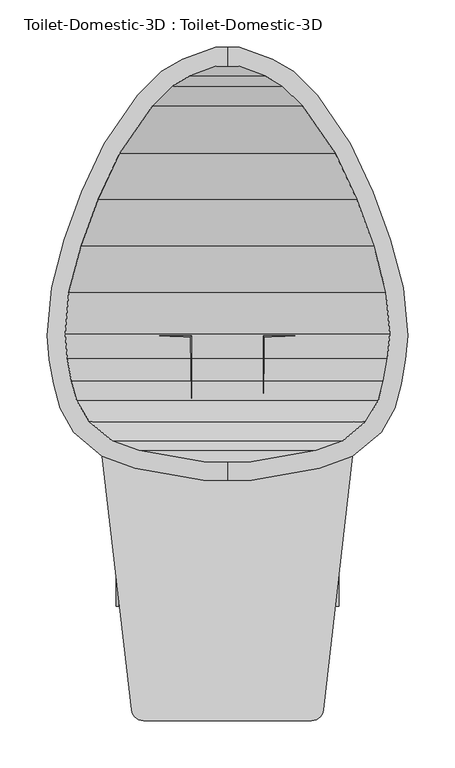
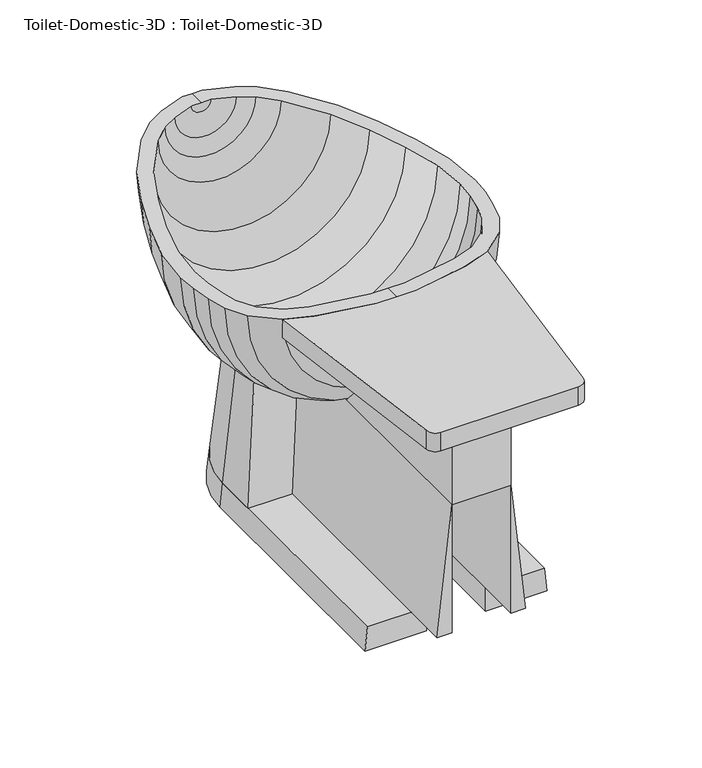
"""IFC4 building model written with IfcOpenShell, lengths in millimetres: flow terminal geometry, Toilet-Domestic-3D : Toilet-Domestic-3D."""

from ifc_helpers import new_model, si_unit, point, frame, frame_2d, origin, place, context, project, spatial, polyline, circle_curve, trimmed, segment, composite_curve, outline, extrude, source, transform, mapped, element, save
from ifc_brep_helpers import plane_surface, revolved_surface, advanced_brep


def toilet_domestic_3d_toilet_domestic_3d_9ecb9d01(model_context):
    return source(origin(), model_context, "Body", "SolidModel", [
        advanced_brep(
        [(-25.4, -152.4, 361.95), (0.0, -152.4, 361.95), (0.0, -133.6394123, 361.95), (-22.0920022, -133.6394123, 361.95), (-94.1172813, -120.9394123, 361.95), (-121.9980886, -110.7916284, 361.95), (-146.1085923, -90.5605136, 361.95), (-159.5484355, -68.2281551, 361.95), (-165.101298, -47.5045901, 361.95), (-169.3087351, -23.6430284, 361.95), (-171.5645445, 2.1409906, 361.95), (-167.7238545, 46.0402777, 361.95), (-154.575847, 95.1093097, 361.95), (-136.654021, 144.3491221, 361.95), (-114.0255101, 192.8761202, 361.95), (-79.2146703, 243.0564036, 361.95), (-58.4178985, 263.8531754, 361.95), (-39.5113323, 274.7688865, 361.95), (-12.5224565, 284.592034, 361.95), (0.0, 284.592034, 361.95), (0.0, 304.8, 361.95), (-12.7, 304.8, 361.95), (-47.5929632, 292.1, 361.95), (-69.5900085, 279.4, 361.95), (-94.9900085, 254.0, 361.95), (-130.2307553, 203.2, 361.95), (-153.9191843, 152.4, 361.95), (-172.4088722, 101.6, 361.95), (-186.0724883, 50.6066907, 361.95), (-190.5, 0.0, 361.95), (-188.2862441, -25.3033453, 361.95), (-183.790496, -50.8, 361.95), (-176.9845865, -76.2, 361.95), (-162.5887836, -101.6, 361.95), (-132.3182423, -127.0, 361.95), (-97.4252791, -139.7, 361.95), (25.4, -152.4, 361.95), (97.4252791, -139.7, 361.95), (132.3182423, -127.0, 361.95), (162.5887836, -101.6, 361.95), (176.9845865, -76.2, 361.95), (183.790496, -50.8, 361.95), (188.2862441, -25.3033453, 361.95), (190.5, 0.0, 361.95), (186.0724883, 50.6066907, 361.95), (172.4088722, 101.6, 361.95), (153.9191843, 152.4, 361.95), (130.2307553, 203.2, 361.95), (94.9900085, 254.0, 361.95), (69.5900085, 279.4, 361.95), (47.5929632, 292.1, 361.95), (12.7, 304.8, 361.95), (12.5224565, 284.592034, 361.95), (39.5113323, 274.7688865, 361.95), (58.4178985, 263.8531754, 361.95), (79.2146703, 243.0564036, 361.95), (114.0255101, 192.8761202, 361.95), (136.654021, 144.3491221, 361.95), (154.575847, 95.1093097, 361.95), (167.7238545, 46.0402777, 361.95), (171.5645445, 2.1409906, 361.95), (169.3087351, -23.6430284, 361.95), (165.101298, -47.5045901, 361.95), (159.5484355, -68.2281551, 361.95), (146.1085923, -90.5605136, 361.95), (121.9980886, -110.7916284, 361.95), (94.1172813, -120.9394123, 361.95), (22.0920022, -133.6394123, 361.95)],
        [
            (0, 1),
            (1, 2),
            (2, 3),
            (3, 4),
            (4, 5),
            (5, 6),
            (6, 7),
            (7, 8),
            (8, 9),
            (9, 10),
            (10, 11),
            (11, 12),
            (12, 13),
            (13, 14),
            (14, 15),
            (15, 16),
            (16, 17),
            (17, 18),
            (18, 19),
            (19, 20),
            (20, 21),
            (21, 22),
            (22, 23),
            (23, 24),
            (24, 25),
            (25, 26),
            (26, 27),
            (27, 28),
            (28, 29),
            (29, 30),
            (30, 31),
            (31, 32),
            (32, 33),
            (33, 34),
            (34, 35),
            (35, 0),
            (36, 37),
            (37, 38),
            (38, 39),
            (39, 40),
            (40, 41),
            (41, 42),
            (42, 43),
            (43, 44),
            (44, 45),
            (45, 46),
            (46, 47),
            (47, 48),
            (48, 49),
            (49, 50),
            (50, 51),
            (51, 20),
            (19, 52),
            (52, 53),
            (53, 54),
            (54, 55),
            (55, 56),
            (56, 57),
            (57, 58),
            (58, 59),
            (59, 60),
            (60, 61),
            (61, 62),
            (62, 63),
            (63, 64),
            (64, 65),
            (65, 66),
            (66, 67),
            (67, 2),
            (1, 36),
            (36, 0, circle_curve(frame((0.0, -152.4, 361.95), z_axis=(0.0, 1.0, 0.0), x_axis=(-1.0, 0.0, 0.0)), 25.4)),
            (35, 37, circle_curve(frame((0.0, -139.7, 361.95), z_axis=(0.0, -1.0, 0.0), x_axis=(-1.0, 0.0, 0.0)), 97.4252791)),
            (34, 38, circle_curve(frame((0.0, -127.0, 361.95), z_axis=(0.0, -1.0, 0.0), x_axis=(-1.0, 0.0, 0.0)), 132.3182423)),
            (33, 39, circle_curve(frame((0.0, -101.6, 361.95), z_axis=(0.0, -1.0, 0.0), x_axis=(-1.0, 0.0, 0.0)), 162.5887836)),
            (32, 40, circle_curve(frame((0.0, -76.2, 361.95), z_axis=(0.0, -1.0, 0.0), x_axis=(-1.0, 0.0, 0.0)), 176.9845865)),
            (31, 41, circle_curve(frame((0.0, -50.8, 361.95), z_axis=(0.0, -1.0, 0.0), x_axis=(-1.0, 0.0, 0.0)), 183.790496)),
            (30, 42, circle_curve(frame((0.0, -25.3033453, 361.95), z_axis=(0.0, -1.0, 0.0), x_axis=(-1.0, 0.0, 0.0)), 188.2862441)),
            (29, 43, circle_curve(frame((0.0, 0.0, 361.95), z_axis=(0.0, -1.0, 0.0), x_axis=(-1.0, 0.0, 0.0)), 190.5)),
            (28, 44, circle_curve(frame((0.0, 50.6066907, 361.95), z_axis=(0.0, -1.0, 0.0), x_axis=(-1.0, 0.0, 0.0)), 186.0724883)),
            (27, 45, circle_curve(frame((0.0, 101.6, 361.95), z_axis=(0.0, -1.0, 0.0), x_axis=(-1.0, 0.0, 0.0)), 172.4088722)),
            (26, 46, circle_curve(frame((0.0, 152.4, 361.95), z_axis=(0.0, -1.0, 0.0), x_axis=(-1.0, 0.0, 0.0)), 153.9191843)),
            (25, 47, circle_curve(frame((0.0, 203.2, 361.95), z_axis=(0.0, -1.0, 0.0), x_axis=(-1.0, 0.0, 0.0)), 130.2307553)),
            (24, 48, circle_curve(frame((0.0, 254.0, 361.95), z_axis=(0.0, -1.0, 0.0), x_axis=(-1.0, 0.0, 0.0)), 94.9900085)),
            (23, 49, circle_curve(frame((0.0, 279.4, 361.95), z_axis=(0.0, -1.0, 0.0), x_axis=(-1.0, 0.0, 0.0)), 69.5900085)),
            (22, 50, circle_curve(frame((0.0, 292.1, 361.95), z_axis=(0.0, -1.0, 0.0), x_axis=(-1.0, 0.0, 0.0)), 47.5929632)),
            (21, 51, circle_curve(frame((0.0, 304.8, 361.95), z_axis=(0.0, -1.0, 0.0), x_axis=(-1.0, 0.0, 0.0)), 12.7)),
            (18, 52, circle_curve(frame((0.0, 284.592034, 361.95), z_axis=(0.0, -1.0, 0.0), x_axis=(-1.0, 0.0, 0.0)), 12.5224565)),
            (17, 53, circle_curve(frame((0.0, 274.7688865, 361.95), z_axis=(0.0, -1.0, 0.0), x_axis=(-1.0, 0.0, 0.0)), 39.5113323)),
            (16, 54, circle_curve(frame((0.0, 263.8531754, 361.95), z_axis=(0.0, -1.0, 0.0), x_axis=(-1.0, 0.0, 0.0)), 58.4178985)),
            (15, 55, circle_curve(frame((0.0, 243.0564036, 361.95), z_axis=(0.0, -1.0, 0.0), x_axis=(-1.0, 0.0, 0.0)), 79.2146703)),
            (14, 56, circle_curve(frame((0.0, 192.8761202, 361.95), z_axis=(0.0, -1.0, 0.0), x_axis=(-1.0, 0.0, 0.0)), 114.0255101)),
            (13, 57, circle_curve(frame((0.0, 144.3491221, 361.95), z_axis=(0.0, -1.0, 0.0), x_axis=(-1.0, 0.0, 0.0)), 136.654021)),
            (12, 58, circle_curve(frame((0.0, 95.1093097, 361.95), z_axis=(0.0, -1.0, 0.0), x_axis=(-1.0, 0.0, 0.0)), 154.575847)),
            (11, 59, circle_curve(frame((0.0, 46.0402777, 361.95), z_axis=(0.0, -1.0, 0.0), x_axis=(-1.0, 0.0, 0.0)), 167.7238545)),
            (10, 60, circle_curve(frame((0.0, 2.1409906, 361.95), z_axis=(0.0, -1.0, 0.0), x_axis=(-1.0, 0.0, 0.0)), 171.5645445)),
            (9, 61, circle_curve(frame((0.0, -23.6430284, 361.95), z_axis=(0.0, -1.0, 0.0), x_axis=(-1.0, 0.0, 0.0)), 169.3087351)),
            (8, 62, circle_curve(frame((0.0, -47.5045901, 361.95), z_axis=(0.0, -1.0, 0.0), x_axis=(-1.0, 0.0, 0.0)), 165.101298)),
            (7, 63, circle_curve(frame((0.0, -68.2281551, 361.95), z_axis=(0.0, -1.0, 0.0), x_axis=(-1.0, 0.0, 0.0)), 159.5484355)),
            (6, 64, circle_curve(frame((0.0, -90.5605136, 361.95), z_axis=(0.0, -1.0, 0.0), x_axis=(-1.0, 0.0, 0.0)), 146.1085923)),
            (5, 65, circle_curve(frame((0.0, -110.7916284, 361.95), z_axis=(0.0, -1.0, 0.0), x_axis=(-1.0, 0.0, 0.0)), 121.9980886)),
            (4, 66, circle_curve(frame((0.0, -120.9394123, 361.95), z_axis=(0.0, -1.0, 0.0), x_axis=(-1.0, 0.0, 0.0)), 94.1172813)),
            (3, 67, circle_curve(frame((0.0, -133.6394123, 361.95), z_axis=(0.0, -1.0, 0.0), x_axis=(-1.0, 0.0, 0.0)), 22.0920022)),
        ],
        [
            plane_surface(frame((0.0, -175.1599017, 361.95), z_axis=(0.0, 0.0, 1.0), x_axis=(-1.0, 0.0, 0.0))),
            plane_surface(frame((0.0, -175.1599017, 361.95), z_axis=(0.0, 0.0, 1.0), x_axis=(1.0, 0.0, 0.0))),
            revolved_surface(polyline([(-25.4, -152.4, 361.95), (-97.4252791, -139.7, 361.95)]), (0.0, -175.1599017, 361.95), (0.0, 1.0, 0.0)),
            revolved_surface(polyline([(-97.4252791, -139.7, 361.95), (-132.3182423, -127.0, 361.95)]), (0.0, -175.1599017, 361.95), (0.0, 1.0, 0.0)),
            revolved_surface(polyline([(-132.3182423, -127.0, 361.95), (-162.5887836, -101.6, 361.95)]), (0.0, -175.1599017, 361.95), (0.0, 1.0, 0.0)),
            revolved_surface(polyline([(-162.5887836, -101.6, 361.95), (-176.9845865, -76.2, 361.95)]), (0.0, -175.1599017, 361.95), (0.0, 1.0, 0.0)),
            revolved_surface(polyline([(-176.9845865, -76.2, 361.95), (-183.790496, -50.8, 361.95)]), (0.0, -175.1599017, 361.95), (0.0, 1.0, 0.0)),
            revolved_surface(polyline([(-183.790496, -50.8, 361.95), (-188.2862441, -25.3033453, 361.95)]), (0.0, -175.1599017, 361.95), (0.0, 1.0, 0.0)),
            revolved_surface(polyline([(-188.2862441, -25.3033453, 361.95), (-190.5, 0.0, 361.95)]), (0.0, -175.1599017, 361.95), (0.0, 1.0, 0.0)),
            revolved_surface(polyline([(-190.5, 0.0, 361.95), (-186.0724883, 50.6066907, 361.95)]), (0.0, -175.1599017, 361.95), (0.0, 1.0, 0.0)),
            revolved_surface(polyline([(-186.0724883, 50.6066907, 361.95), (-172.4088722, 101.6, 361.95)]), (0.0, -175.1599017, 361.95), (0.0, 1.0, 0.0)),
            revolved_surface(polyline([(-172.4088722, 101.6, 361.95), (-153.9191843, 152.4, 361.95)]), (0.0, -175.1599017, 361.95), (0.0, 1.0, 0.0)),
            revolved_surface(polyline([(-153.9191843, 152.4, 361.95), (-130.2307553, 203.2, 361.95)]), (0.0, -175.1599017, 361.95), (0.0, 1.0, 0.0)),
            revolved_surface(polyline([(-130.2307553, 203.2, 361.95), (-94.9900085, 254.0, 361.95)]), (0.0, -175.1599017, 361.95), (0.0, 1.0, 0.0)),
            revolved_surface(polyline([(-94.9900085, 254.0, 361.95), (-69.5900085, 279.4, 361.95)]), (0.0, -175.1599017, 361.95), (0.0, 1.0, 0.0)),
            revolved_surface(polyline([(-69.5900085, 279.4, 361.95), (-47.5929632, 292.1, 361.95)]), (0.0, -175.1599017, 361.95), (0.0, 1.0, 0.0)),
            revolved_surface(polyline([(-47.5929632, 292.1, 361.95), (-12.7, 304.8, 361.95)]), (0.0, -175.1599017, 361.95), (0.0, 1.0, 0.0)),
            plane_surface(frame((0.0, 304.8, 361.95), z_axis=(0.0, 1.0, 0.0), x_axis=(-1.0, 0.0, 0.0))),
            plane_surface(frame((0.0, 284.592034, 361.95), z_axis=(0.0, -1.0, 0.0), x_axis=(-1.0, 0.0, 0.0))),
            revolved_surface(polyline([(-12.5224565, 284.592034, 361.95), (-39.5113323, 274.7688865, 361.95)]), (0.0, -175.1599017, 361.95), (0.0, 1.0, 0.0)),
            revolved_surface(polyline([(-39.5113323, 274.7688865, 361.95), (-58.4178985, 263.8531754, 361.95)]), (0.0, -175.1599017, 361.95), (0.0, 1.0, 0.0)),
            revolved_surface(polyline([(-58.4178985, 263.8531754, 361.95), (-79.2146703, 243.0564036, 361.95)]), (0.0, -175.1599017, 361.95), (0.0, 1.0, 0.0)),
            revolved_surface(polyline([(-79.2146703, 243.0564036, 361.95), (-114.0255101, 192.8761202, 361.95)]), (0.0, -175.1599017, 361.95), (0.0, 1.0, 0.0)),
            revolved_surface(polyline([(-114.0255101, 192.8761202, 361.95), (-136.654021, 144.3491221, 361.95)]), (0.0, -175.1599017, 361.95), (0.0, 1.0, 0.0)),
            revolved_surface(polyline([(-136.654021, 144.3491221, 361.95), (-154.575847, 95.1093097, 361.95)]), (0.0, -175.1599017, 361.95), (0.0, 1.0, 0.0)),
            revolved_surface(polyline([(-154.575847, 95.1093097, 361.95), (-167.7238545, 46.0402777, 361.95)]), (0.0, -175.1599017, 361.95), (0.0, 1.0, 0.0)),
            revolved_surface(polyline([(-167.7238545, 46.0402777, 361.95), (-171.5645445, 2.1409906, 361.95)]), (0.0, -175.1599017, 361.95), (0.0, 1.0, 0.0)),
            revolved_surface(polyline([(-171.5645445, 2.1409906, 361.95), (-169.3087351, -23.6430284, 361.95)]), (0.0, -175.1599017, 361.95), (0.0, 1.0, 0.0)),
            revolved_surface(polyline([(-169.3087351, -23.6430284, 361.95), (-165.101298, -47.5045901, 361.95)]), (0.0, -175.1599017, 361.95), (0.0, 1.0, 0.0)),
            revolved_surface(polyline([(-165.101298, -47.5045901, 361.95), (-159.5484355, -68.2281551, 361.95)]), (0.0, -175.1599017, 361.95), (0.0, 1.0, 0.0)),
            revolved_surface(polyline([(-159.5484355, -68.2281551, 361.95), (-146.1085923, -90.5605136, 361.95)]), (0.0, -175.1599017, 361.95), (0.0, 1.0, 0.0)),
            revolved_surface(polyline([(-146.1085923, -90.5605136, 361.95), (-121.9980886, -110.7916284, 361.95)]), (0.0, -175.1599017, 361.95), (0.0, 1.0, 0.0)),
            revolved_surface(polyline([(-121.9980886, -110.7916284, 361.95), (-94.1172813, -120.9394123, 361.95)]), (0.0, -175.1599017, 361.95), (0.0, 1.0, 0.0)),
            revolved_surface(polyline([(-94.1172813, -120.9394123, 361.95), (-22.0920022, -133.6394123, 361.95)]), (0.0, -175.1599017, 361.95), (0.0, 1.0, 0.0)),
            plane_surface(frame((0.0, -133.6394123, 361.95), z_axis=(0.0, 1.0, 0.0), x_axis=(-1.0, 0.0, 0.0))),
            plane_surface(frame((0.0, -152.4, 361.95), z_axis=(0.0, -1.0, 0.0), x_axis=(-1.0, 0.0, 0.0))),
        ],
        [
            (0, [[1, 2, 3, 4, 5, 6, 7, 8, 9, 10, 11, 12, 13, 14, 15, 16, 17, 18, 19, 20, 21, 22, 23, 24, 25, 26, 27, 28, 29, 30, 31, 32, 33, 34, 35, 36]]),
            (1, [[37, 38, 39, 40, 41, 42, 43, 44, 45, 46, 47, 48, 49, 50, 51, 52, -20, 53, 54, 55, 56, 57, 58, 59, 60, 61, 62, 63, 64, 65, 66, 67, 68, 69, -2, 70]]),
            (2, [[-37, 71, -36, 72]]),
            (3, [[-38, -72, -35, 73]]),
            (4, [[-39, -73, -34, 74]]),
            (5, [[-40, -74, -33, 75]]),
            (6, [[-41, -75, -32, 76]]),
            (7, [[-42, -76, -31, 77]]),
            (8, [[-43, -77, -30, 78]]),
            (9, [[-44, -78, -29, 79]]),
            (10, [[-45, -79, -28, 80]]),
            (11, [[-46, -80, -27, 81]]),
            (12, [[-47, -81, -26, 82]]),
            (13, [[-48, -82, -25, 83]]),
            (14, [[-49, -83, -24, 84]]),
            (15, [[-50, -84, -23, 85]]),
            (16, [[-51, -85, -22, 86]]),
            (17, [[-52, -86, -21]]),
            (18, [[-53, -19, 87]]),
            (19, [[-54, -87, -18, 88]]),
            (20, [[-55, -88, -17, 89]]),
            (21, [[-56, -89, -16, 90]]),
            (22, [[-57, -90, -15, 91]]),
            (23, [[-58, -91, -14, 92]]),
            (24, [[-59, -92, -13, 93]]),
            (25, [[-60, -93, -12, 94]]),
            (26, [[-61, -94, -11, 95]]),
            (27, [[-62, -95, -10, 96]]),
            (28, [[-63, -96, -9, 97]]),
            (29, [[-64, -97, -8, 98]]),
            (30, [[-65, -98, -7, 99]]),
            (31, [[-66, -99, -6, 100]]),
            (32, [[-67, -100, -5, 101]]),
            (33, [[-68, -101, -4, 102]]),
            (34, [[-69, -102, -3]]),
            (35, [[-70, -1, -71]]),
        ],
    ),
        advanced_brep(
        [(-57.15, -342.9, 31.75), (-38.1, -342.9, 31.75), (-38.1, -342.9, 206.375), (-38.1, 0.0, 206.375), (-57.15, -19.05, 31.75), (-38.1, 0.0, 31.75), (-95.25, 0.0, 206.375), (-114.3, -19.05, 31.75), (-95.25, 0.0, 31.75), (-95.25, 38.1, 206.375), (-114.3, 38.1, 31.75), (-95.25, 38.1, 31.75), (95.25, 38.1, 206.375), (114.3, 38.1, 31.75), (95.25, 38.1, 31.75), (95.25, 0.0, 206.375), (114.3, -19.05, 31.75), (95.25, 0.0, 31.75), (38.1, 0.0, 206.375), (57.15, -19.05, 31.75), (38.1, 0.0, 31.75), (57.15, -342.9, 31.75), (38.1, -342.9, 206.375), (38.1, -342.9, 31.75)],
        [
            (0, 1),
            (1, 2),
            (2, 0),
            (2, 3),
            (3, 4),
            (4, 0),
            (1, 5),
            (5, 3),
            (4, 5),
            (3, 6),
            (6, 7),
            (7, 4),
            (5, 8),
            (8, 6),
            (7, 8),
            (6, 9),
            (9, 10),
            (10, 7),
            (8, 11),
            (11, 9),
            (10, 11),
            (12, 13),
            (13, 10, circle_curve(frame((0.0, 38.1, 31.75), z_axis=(0.0, 0.0, 1.0), x_axis=(-1.0, 0.0, 0.0)), 114.3)),
            (9, 12, circle_curve(frame((0.0, 38.1, 206.375), z_axis=(0.0, 0.0, -1.0), x_axis=(-1.0, 0.0, 0.0)), 95.25)),
            (14, 12),
            (11, 14, circle_curve(frame((0.0, 38.1, 31.75), z_axis=(0.0, 0.0, -1.0), x_axis=(-1.0, 0.0, 0.0)), 95.25)),
            (13, 14),
            (12, 15),
            (15, 16),
            (16, 13),
            (14, 17),
            (17, 15),
            (16, 17),
            (15, 18),
            (18, 19),
            (19, 16),
            (17, 20),
            (20, 18),
            (19, 20),
            (21, 22),
            (22, 23),
            (23, 21),
            (18, 22),
            (21, 19),
            (20, 23),
        ],
        [
            plane_surface(frame((-244.475, -342.9, 0.0), z_axis=(0.0, -1.0, 0.0), x_axis=(0.0, 0.0, -1.0))),
            plane_surface(frame((-57.15, -342.9, 31.75), z_axis=(-0.9941021766079944, 0.0, 0.10844751017542063), x_axis=(0.0, 1.0, 0.0))),
            plane_surface(frame((-38.1, -342.9, 206.375), z_axis=(1.0, 0.0, 0.0), x_axis=(0.0, 1.0, 0.0))),
            plane_surface(frame((-38.1, -342.9, 31.75), z_axis=(0.0, 0.0, -1.0), x_axis=(0.0, 1.0, 0.0))),
            plane_surface(frame((-57.15, -19.05, 31.75), z_axis=(0.0, -0.9941021766079944, 0.10844751017542063), x_axis=(-1.0, 0.0, 0.0))),
            plane_surface(frame((-38.1, 0.0, 206.375), z_axis=(0.0, 1.0, 0.0), x_axis=(-1.0, 0.0, 0.0))),
            plane_surface(frame((-38.1, 0.0, 31.75), z_axis=(0.0, 0.0, -1.0), x_axis=(-1.0, 0.0, 0.0))),
            plane_surface(frame((-114.3, -19.05, 31.75), z_axis=(-0.9941021766079944, 0.0, 0.10844751017542063), x_axis=(0.0, 1.0, 0.0))),
            plane_surface(frame((-95.25, 0.0, 206.375), z_axis=(1.0, 0.0, 0.0), x_axis=(0.0, 1.0, 0.0))),
            plane_surface(frame((-95.25, 0.0, 31.75), z_axis=(0.0, 0.0, -1.0), x_axis=(0.0, 1.0, 0.0))),
            revolved_surface(polyline([(-114.3, 38.1, 31.75), (-95.25, 38.1, 206.375)]), (0.0, 38.1, 0.0), (0.0, 0.0, 1.0)),
            revolved_surface(polyline([(-95.25, 38.1, 206.375), (-95.25, 38.1, 31.75)]), (0.0, 38.1, 0.0), (0.0, 0.0, 1.0)),
            plane_surface(frame((0.0, 38.1, 31.75), z_axis=(0.0, 0.0, -1.0), x_axis=(-1.0, 0.0, 0.0))),
            plane_surface(frame((114.3, 38.1, 31.75), z_axis=(0.9941021766079944, 0.0, 0.10844751017542063), x_axis=(0.0, -1.0, 0.0))),
            plane_surface(frame((95.25, 38.1, 206.375), z_axis=(-1.0, 0.0, 0.0), x_axis=(0.0, -1.0, 0.0))),
            plane_surface(frame((95.25, 38.1, 31.75), z_axis=(0.0, 0.0, -1.0), x_axis=(0.0, -1.0, 0.0))),
            plane_surface(frame((114.3, -19.05, 31.75), z_axis=(0.0, -0.9941021766079944, 0.10844751017542063), x_axis=(-1.0, 0.0, 0.0))),
            plane_surface(frame((95.25, 0.0, 206.375), z_axis=(0.0, 1.0, 0.0), x_axis=(-1.0, 0.0, 0.0))),
            plane_surface(frame((95.25, 0.0, 31.75), z_axis=(0.0, 0.0, -1.0), x_axis=(-1.0, 0.0, 0.0))),
            plane_surface(frame((-168.275, -342.9, 0.0), z_axis=(0.0, -1.0, 0.0), x_axis=(0.0, 0.0, 1.0))),
            plane_surface(frame((57.15, -19.05, 31.75), z_axis=(0.9941021766079944, 0.0, 0.10844751017542063), x_axis=(0.0, -1.0, 0.0))),
            plane_surface(frame((38.1, 0.0, 206.375), z_axis=(-1.0, 0.0, 0.0), x_axis=(0.0, -1.0, 0.0))),
            plane_surface(frame((38.1, 0.0, 31.75), z_axis=(0.0, 0.0, -1.0), x_axis=(0.0, -1.0, 0.0))),
        ],
        [
            (0, [[1, 2, 3]]),
            (1, [[4, 5, 6, -3]]),
            (2, [[7, 8, -4, -2]]),
            (3, [[-6, 9, -7, -1]]),
            (4, [[10, 11, 12, -5]]),
            (5, [[13, 14, -10, -8]]),
            (6, [[-12, 15, -13, -9]]),
            (7, [[16, 17, 18, -11]]),
            (8, [[19, 20, -16, -14]]),
            (9, [[-18, 21, -19, -15]]),
            (10, [[22, 23, -17, 24]]),
            (11, [[25, -24, -20, 26]]),
            (12, [[27, -26, -21, -23]]),
            (13, [[28, 29, 30, -22]]),
            (14, [[31, 32, -28, -25]]),
            (15, [[-30, 33, -31, -27]]),
            (16, [[34, 35, 36, -29]]),
            (17, [[37, 38, -34, -32]]),
            (18, [[-36, 39, -37, -33]]),
            (19, [[40, 41, 42]]),
            (20, [[43, -40, 44, -35]]),
            (21, [[45, -41, -43, -38]]),
            (22, [[-44, -42, -45, -39]]),
        ],
    ),
        advanced_brep(
        [(-117.7636364, -285.75, 0.0), (-38.1, -285.75, 0.0), (-38.1, -285.75, 31.75), (-114.3, -285.75, 31.75), (-114.3, 38.0999951, 31.75), (-117.7636364, 38.0999951, 0.0), (-38.1, 38.0999951, 31.75), (-38.1, 38.0999951, 0.0), (114.2999707, 38.0999951, 31.75), (117.7636071, 38.0999951, 0.0), (38.0999707, 38.0999951, 31.75), (38.0999707, 38.0999951, 0.0), (117.7636071, -285.6681634, 0.0), (114.2999707, -285.6681634, 31.75), (38.0999707, -285.6681634, 31.75), (38.0999707, -285.6681634, 0.0)],
        [
            (0, 1),
            (1, 2),
            (2, 3),
            (3, 0),
            (3, 4),
            (4, 5),
            (5, 0),
            (2, 6),
            (6, 4),
            (1, 7),
            (7, 6),
            (5, 7),
            (8, 9),
            (9, 5, circle_curve(frame((-1.46e-05, 38.0999951, 0.0), z_axis=(0.0, 0.0, 1.0), x_axis=(-1.0, 0.0, 0.0)), 117.7636217)),
            (4, 8, circle_curve(frame((-1.46e-05, 38.0999951, 31.75), z_axis=(0.0, 0.0, -1.0), x_axis=(-1.0, 0.0, 0.0)), 114.2999854)),
            (10, 8),
            (6, 10, circle_curve(frame((-1.46e-05, 38.0999951, 31.75), z_axis=(0.0, 0.0, -1.0), x_axis=(-1.0, 0.0, 0.0)), 38.0999854)),
            (11, 10),
            (7, 11, circle_curve(frame((-1.46e-05, 38.0999951, 0.0), z_axis=(0.0, 0.0, -1.0), x_axis=(-1.0, 0.0, 0.0)), 38.0999854)),
            (9, 11),
            (12, 13),
            (13, 14),
            (14, 15),
            (15, 12),
            (8, 13),
            (12, 9),
            (10, 14),
            (11, 15),
        ],
        [
            plane_surface(frame((-196.85, -285.75, 0.0), z_axis=(0.0, -1.0, 0.0), x_axis=(0.0, 0.0, -1.0))),
            plane_surface(frame((-117.7636364, -285.75, 0.0), z_axis=(-0.9941021766079929, 0.0, 0.10844751017543448), x_axis=(0.0, 1.0, 0.0))),
            plane_surface(frame((-114.3, -285.75, 31.75), z_axis=(0.0, 0.0, 1.0), x_axis=(0.0, 1.0, 0.0))),
            plane_surface(frame((-38.1, -285.75, 31.75), z_axis=(1.0, 0.0, 0.0), x_axis=(0.0, 1.0, 0.0))),
            plane_surface(frame((-38.1, -285.75, 0.0), z_axis=(0.0, 0.0, -1.0), x_axis=(0.0, 1.0, 0.0))),
            revolved_surface(polyline([(-117.7636364, 38.0999951, 0.0), (-114.3, 38.0999951, 31.75)]), (-1.46e-05, 38.0999951, 0.0), (0.0, 0.0, 1.0)),
            plane_surface(frame((-1.46e-05, 38.0999951, 31.75), z_axis=(0.0, 0.0, 1.0), x_axis=(-1.0, 0.0, 0.0))),
            revolved_surface(polyline([(-38.1, 38.0999951, 31.75), (-38.1, 38.0999951, 0.0)]), (-1.46e-05, 38.0999951, 0.0), (0.0, 0.0, 1.0)),
            plane_surface(frame((-1.46e-05, 38.0999951, 0.0), z_axis=(0.0, 0.0, -1.0), x_axis=(-1.0, 0.0, 0.0))),
            plane_surface(frame((31.7499707, -285.6681634, 0.0), z_axis=(0.0, -1.0, 0.0), x_axis=(0.0, 0.0, 1.0))),
            plane_surface(frame((117.7636071, 38.0999951, 0.0), z_axis=(0.9941021766079929, 0.0, 0.10844751017543448), x_axis=(0.0, -1.0, 0.0))),
            plane_surface(frame((114.2999707, 38.0999951, 31.75), z_axis=(0.0, 0.0, 1.0), x_axis=(0.0, -1.0, 0.0))),
            plane_surface(frame((38.0999707, 38.0999951, 31.75), z_axis=(-1.0, 0.0, 0.0), x_axis=(0.0, -1.0, 0.0))),
            plane_surface(frame((38.0999707, 38.0999951, 0.0), z_axis=(0.0, 0.0, -1.0), x_axis=(0.0, -1.0, 0.0))),
        ],
        [
            (0, [[1, 2, 3, 4]]),
            (1, [[5, 6, 7, -4]]),
            (2, [[8, 9, -5, -3]]),
            (3, [[10, 11, -8, -2]]),
            (4, [[-7, 12, -10, -1]]),
            (5, [[13, 14, -6, 15]]),
            (6, [[16, -15, -9, 17]]),
            (7, [[18, -17, -11, 19]]),
            (8, [[20, -19, -12, -14]]),
            (9, [[21, 22, 23, 24]]),
            (10, [[25, -21, 26, -13]]),
            (11, [[27, -22, -25, -16]]),
            (12, [[28, -23, -27, -18]]),
            (13, [[-26, -24, -28, -20]]),
        ],
    ),
        extrude(outline(polyline([(-139.7, 264.5247209), (-127.0, 229.6317577), (-107.4852632, 206.375), (-342.9, 206.375), (-342.9, 336.55), (-152.4, 336.55), (-139.7, 264.5247209)])), frame((-38.1, 0.0, 0.0), z_axis=(1.0, 0.0, 0.0), x_axis=(0.0, 1.0, 0.0)), (0.0, 0.0, 1.0), 76.2),
        extrude(outline(composite_curve([segment(polyline([(-25.4, -152.4), (0.0, -152.4), (25.4, -152.4), (97.4252791, -139.7), (132.3182423, -127.0), (101.4824733, -395.1508638)]), True, "CONTINUOUS"), segment(trimmed(circle_curve(frame_2d((88.8656197, -393.7)), 12.7), [point((101.4824733, -395.1508638))], [point((88.8656197, -406.4))], False, "CARTESIAN"), True, "CONTINUOUS"), segment(polyline([(88.8656197, -406.4), (-88.8656197, -406.4)]), True, "CONTINUOUS"), segment(trimmed(circle_curve(frame_2d((-88.8656197, -393.7)), 12.7), [point((-88.8656197, -406.4))], [point((-101.4824733, -395.1508638))], False, "CARTESIAN"), True, "CONTINUOUS"), segment(polyline([(-101.4824733, -395.1508638), (-132.3182423, -127.0), (-97.4252791, -139.7), (-25.4, -152.4)]), True, "CONTINUOUS")], self_intersect=False)), frame((0.0, 0.0, 336.55), z_axis=(0.0, 0.0, 1.0), x_axis=(1.0, 0.0, 0.0)), (0.0, 0.0, 1.0), 25.4),
    ])


if __name__ == "__main__":
    model = new_model("IFC4")
    model_context = context("Model", 3, world=origin())
    ifc_project = project(units=[si_unit("LENGTHUNIT", "METRE", prefix="MILLI")], contexts=[model_context])
    site = spatial("IfcSite", under=ifc_project)
    building = spatial("IfcBuilding", under=site)
    placement = place(None, origin())
    toilet_domestic_3d_toilet_domestic_3d_shape = toilet_domestic_3d_toilet_domestic_3d_9ecb9d01(model_context)
    element("IfcFlowTerminal", 1, ObjectType="Toilet-Domestic-3D : Toilet-Domestic-3D", at=placement, inside=building, context=model_context, shape_type="MappedRepresentation", body=[
        mapped(toilet_domestic_3d_toilet_domestic_3d_shape, transform((0.0, 0.0, 0.0), x_axis=(1.0, 0.0, 0.0), y_axis=(0.0, 1.0, 0.0), z_axis=(0.0, 0.0, 1.0))),
    ])
    save(model, "model.ifc")

# Revit data of these elements
# Type "Toilet-Domestic-3D : Toilet-Domestic-3D"
#   Assembly Code = "D2010110"
#   Toilet - Bowl/Basin Material = Porcelain, Linen
#   Toilet - Seat Material = Laminate, Linen, Matte
#   Default Elevation = 0
# Element 1 (IfcFlowTerminal, "Toilet-Domestic-3D : Toilet-Domestic-3D")
#   Materials on its faces: "Porcelain, Linen", "Laminate, Linen, Matte"
# Materials
#   "Porcelain, Linen": class "Ceramic", colour RGB 249 239 230, transparency 0, Description = "Porcelain, linen", Cost = 0
#   "Laminate, Linen, Matte": class "Plastic", colour RGB 249 239 230, transparency 0, Description = "Plastic Laminate - Linen, Matte", Cost = 0
